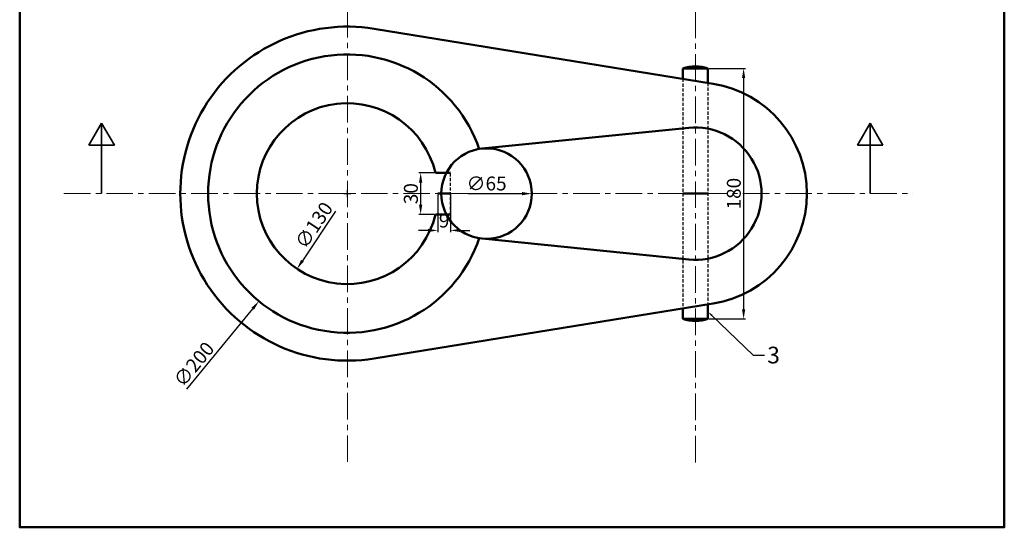
# Model space of a CAD drawing. Units: millimetres. Extents: x 1219 to 1926, y 574 to 1498.
# Tile 1 of 2: x 1219 to 1926, y 574 to 938. Entities that reach past the tile are written whole.
import ezdxf
from ezdxf import colors
from ezdxf.entities.mleader import LeaderData, LeaderLine
from ezdxf.math import Vec2, Vec3

# ---------------------------------------------------------------- set-up
doc = ezdxf.new("R2010")
doc.units = ezdxf.units.MM
doc.header["$LTSCALE"] = 0.6
doc.linetypes.add('CENTER', pattern=[50.8, 31.75, -6.35, 6.35, -6.35])
doc.linetypes.add('HIDDEN', pattern=[9.525, 6.35, -3.175])
for name, color, linetype, lineweight in [('M-CNTR', 1, 'CENTER', 18), ('M-DIMS', 2, 'Continuous', 25), ('M-HIDN', 6, 'HIDDEN', 25), ('M-OUTL', 7, 'Continuous', 50), ('M-SECT', 4, 'Continuous', 35), ('M-TEXT', 3, 'Continuous', 25), ('M-TTLB', 7, 'Continuous', 50)]:
    doc.layers.add(name, color=color, linetype=linetype, lineweight=lineweight)
doc.styles.get("Standard").update_dxf_attribs({"font": 'arial.ttf'})
doc.dimstyles.new('ISO-25', dxfattribs={"dimtxt": 10, "dimasz": 7, "dimexe": 1.25, "dimexo": 0.625, "dimtad": 1, "dimdec": 0, "dimtxsty": 'Standard', "dimcen": 2.5, "dimadec": 0, "dimazin": 0, "dimtfac": 1, "dimtdec": 0, "dimtofl": 0, "dimtmove": 0, "dimatfit": 3, "dimfxl": 1, "dimarcsym": 0})

# ---------------------------------------------------------------- blocks, each defined once
blk = doc.blocks.new('*D28')
at = {"layer": 'Defpoints', "color": 0, "ltscale": 0.6, "transparency": 16777216}
for p in [(1712.94, 903.44), (1712.94, 723.44), (1738.54, 723.44)]:
    blk.add_point(p, dxfattribs=at)
at = {"layer": 'M-DIMS', "color": 0, "lineweight": -2, "ltscale": 0.6, "transparency": 16777216}
for p, q in [((1713.57, 903.44), (1739.79, 903.44)), ((1738.54, 896.44), (1738.54, 730.44)), ((1713.57, 723.44), (1739.79, 723.44))]:
    blk.add_line(p, q, dxfattribs=at)
at = {"layer": 'M-DIMS', "color": 0, "ltscale": 0.6, "transparency": 16777216}
for points in [[(1737.37, 896.44), (1739.7, 896.44), (1738.54, 903.44)], [(1737.37, 730.44), (1739.7, 730.44), (1738.54, 723.44)]]:
    blk.add_solid(points, dxfattribs=at)
at = {"layer": 'M-DIMS', "color": 0, "ltscale": 0.6, "transparency": 16777216, "insert": (1732.8, 813.44), "char_height": 10, "attachment_point": 5, "rotation": 90}
blk.add_mtext('180', dxfattribs=at)
blk = doc.blocks.new('*D29')
at = {"layer": 'Defpoints', "color": 0, "ltscale": 0.6, "transparency": 16777216}
for p in [(1517.43, 890.7), (1390.45, 736.18)]:
    blk.add_point(p, dxfattribs=at)
at = {"layer": 'M-DIMS', "color": 0, "lineweight": -2, "ltscale": 0.6, "transparency": 16777216}
for p, q in [((1451.44, 813.44), (1456.44, 813.44)), ((1453.94, 810.94), (1453.94, 815.94)), ((1338.55, 673.02), (1386.01, 730.77))]:
    blk.add_line(p, q, dxfattribs=at)
at = {"layer": 'M-DIMS', "color": 0, "ltscale": 0.6, "transparency": 16777216}
blk.add_solid([(1385.11, 731.51), (1386.91, 730.03), (1390.45, 736.18)], dxfattribs=at)
at = {"layer": 'M-DIMS', "color": 0, "ltscale": 0.6, "transparency": 16777216, "insert": (1344.76, 690.04), "char_height": 10, "attachment_point": 5, "rotation": 50.58839}
blk.add_mtext('∅200', dxfattribs=at)
blk = doc.blocks.new('*D30')
at = {"layer": 'Defpoints', "color": 0, "ltscale": 0.6, "transparency": 16777216}
for p in [(1490.08, 867.47), (1417.8, 759.41)]:
    blk.add_point(p, dxfattribs=at)
at = {"layer": 'M-DIMS', "color": 0, "lineweight": -2, "ltscale": 0.6, "transparency": 16777216}
blk.add_line((1445.55, 800.9), (1421.7, 765.23), dxfattribs=at)
at = {"layer": 'M-DIMS', "color": 0, "ltscale": 0.6, "transparency": 16777216}
blk.add_solid([(1420.73, 765.88), (1422.67, 764.58), (1417.8, 759.41)], dxfattribs=at)
at = {"layer": 'M-DIMS', "color": 0, "ltscale": 0.6, "transparency": 16777216, "insert": (1431.05, 790.03), "char_height": 10, "attachment_point": 5, "rotation": 56.22166}
blk.add_mtext('∅130', dxfattribs=at)
blk = doc.blocks.new('*D31')
at = {"layer": 'Defpoints', "color": 0, "ltscale": 0.6, "transparency": 16777216}
for p in [(1521.44, 813.44), (1586.44, 813.44)]:
    blk.add_point(p, dxfattribs=at)
at = {"layer": 'M-DIMS', "color": 0, "lineweight": -2, "ltscale": 0.6, "transparency": 16777216}
blk.add_line((1540.68, 813.44), (1579.44, 813.44), dxfattribs=at)
at = {"layer": 'M-DIMS', "color": 0, "ltscale": 0.6, "transparency": 16777216}
blk.add_solid([(1579.44, 814.61), (1579.44, 812.27), (1586.44, 813.44)], dxfattribs=at)
at = {"layer": 'M-DIMS', "color": 0, "ltscale": 0.6, "transparency": 16777216, "insert": (1553.94, 819.45), "char_height": 10, "attachment_point": 5}
blk.add_mtext('∅65', dxfattribs=at)
blk = doc.blocks.new('*D32')
at = {"layer": 'Defpoints', "color": 0, "ltscale": 0.6, "transparency": 16777216}
for p in [(1517.19, 828.44), (1506.6, 798.44), (1517.19, 798.44)]:
    blk.add_point(p, dxfattribs=at)
at = {"layer": 'M-DIMS', "color": 0, "lineweight": -2, "ltscale": 0.6, "transparency": 16777216}
for p, q in [((1516.56, 828.44), (1505.35, 828.44)), ((1506.6, 821.44), (1506.6, 805.44)), ((1516.56, 798.44), (1505.35, 798.44))]:
    blk.add_line(p, q, dxfattribs=at)
at = {"layer": 'M-DIMS', "color": 0, "ltscale": 0.6, "transparency": 16777216}
for points in [[(1505.43, 821.44), (1507.76, 821.44), (1506.6, 828.44)], [(1505.43, 805.44), (1507.76, 805.44), (1506.6, 798.44)]]:
    blk.add_solid(points, dxfattribs=at)
at = {"layer": 'M-DIMS', "color": 0, "ltscale": 0.6, "transparency": 16777216, "insert": (1500.86, 813.44), "char_height": 10, "attachment_point": 5, "rotation": 90}
blk.add_mtext('30', dxfattribs=at)
blk = doc.blocks.new('*D33')
at = {"layer": 'Defpoints', "color": 0, "ltscale": 0.6, "transparency": 16777216}
for p in [(1518.94, 813.44), (1527.94, 813.44), (1527.94, 787.03)]:
    blk.add_point(p, dxfattribs=at)
at = {"layer": 'M-DIMS', "color": 0, "lineweight": -2, "ltscale": 0.6, "transparency": 16777216}
for p, q in [((1518.94, 812.81), (1518.94, 785.78)), ((1527.94, 812.81), (1527.94, 785.78)), ((1511.94, 787.03), (1504.94, 787.03)), ((1534.94, 787.03), (1541.94, 787.03))]:
    blk.add_line(p, q, dxfattribs=at)
at = {"layer": 'M-DIMS', "color": 0, "ltscale": 0.6, "transparency": 16777216}
for points in [[(1511.94, 788.2), (1511.94, 785.87), (1518.94, 787.03)], [(1534.94, 788.2), (1534.94, 785.87), (1527.94, 787.03)]]:
    blk.add_solid(points, dxfattribs=at)
at = {"layer": 'M-DIMS', "color": 0, "ltscale": 0.6, "transparency": 16777216, "insert": (1523.44, 792.77), "char_height": 10, "attachment_point": 5}
blk.add_mtext('9', dxfattribs=at)
blk = doc.blocks.new('SECTION-ARROW')
at = {"ltscale": 0.6}
for p, q in [((9.14, 50.7), (0, 34.87)), ((9.14, 0), (9.14, 50.7)), ((9.14, 50.7), (18.28, 34.87)), ((0, 34.87), (18.28, 34.87))]:
    blk.add_line(p, q, dxfattribs=at)

msp = doc.modelspace()

# ---------------------------------------------------------------- linework, layer by layer
at = {"layer": 'M-CNTR'}
for p, q in [((1703.94, 620.33), (1703.94, 1419.58)), ((1453.94, 620.73), (1453.94, 1146.58)), ((1250.4, 813.44), (1860.03, 813.44))]:
    msp.add_line(p, q, dxfattribs=at)
at = {"layer": 'M-HIDN', "ltscale": 0.6}
for p, q in [((1694.94, 895.94), (1694.94, 730.94)), ((1712.94, 893.02), (1712.94, 734.47)), ((1527.94, 798.44), (1527.94, 828.44))]:
    msp.add_line(p, q, dxfattribs=at)
at = {"layer": 'M-OUTL'}
for p, q in [((1473.14, 931.89), (1716.74, 892.41)), ((1473.14, 694.98), (1716.74, 734.47))]:
    msp.add_line(p, q, dxfattribs=at)
at = {"layer": 'M-OUTL', "ltscale": 0.6}
for p, q in [((1694.94, 903.44), (1694.94, 895.94)), ((1712.94, 903.44), (1694.94, 903.44)), ((1712.94, 893.02), (1712.94, 903.44)), ((1699.19, 860.7), (1550.69, 845.78)), ((1517.19, 828.44), (1527.94, 828.44)), ((1518.94, 813.44), (1527.94, 813.44)), ((1694.94, 813.44), (1712.94, 813.44)), ((1517.19, 798.44), (1527.94, 798.44)), ((1699.19, 766.18), (1550.69, 781.1)), ((1694.94, 730.94), (1694.94, 723.44)), ((1712.94, 723.44), (1712.94, 733.85)), ((1694.94, 723.44), (1712.94, 723.44))]:
    msp.add_line(p, q, dxfattribs=at)
msp.add_circle((1553.94, 813.44), 32.5, dxfattribs=at)
at = {"layer": 'M-OUTL'}
for centre, radius, start, end in [((1453.94, 813.44), 120, 80.7931, 279.2069), ((1453.94, 813.44), 100, 18.70407, 341.29593), ((1703.94, 813.44), 80, 279.2069, 80.7931), ((1453.94, 813.44), 65, 13.34236, 346.65764)]:
    msp.add_arc(centre, radius, start, end, dxfattribs=at)
at = {"layer": 'M-OUTL', "ltscale": 0.6}
for centre, radius, start, end in [((1703.94, 877.7), 27.27, 70.72588, 109.27412), ((1703.94, 813.44), 47.5, 264.26083, 95.73917), ((1703.94, 749.18), 27.27, 250.72588, 289.27412)]:
    msp.add_arc(centre, radius, start, end, dxfattribs=at)
at = {"layer": 'M-TTLB', "ltscale": 0.6}
msp.add_lwpolyline([(1218.63, 1497.51), (1925.77, 1497.51), (1925.77, 573.72), (1218.63, 573.72)], close=True, dxfattribs=at)

# ---------------------------------------------------------------- block references
at = {"layer": 'M-SECT'}
for p in [(1268.34, 813.44), (1820.28, 813.44)]:
    msp.add_blockref('SECTION-ARROW', p, dxfattribs=at)

# ---------------------------------------------------------------- dimensions: what is measured, and where the dimension line sits
at = {"layer": 'M-DIMS', "ltscale": 0.6}
for base, p1, p2, picture, middle in [((1738.54, 723.44), (1712.94, 903.44), (1712.94, 723.44), '*D28', (1732.8, 813.44)), ((1506.6, 798.44), (1517.19, 828.44), (1517.19, 798.44), '*D32', (1500.86, 813.44))]:
    dim = msp.add_linear_dim(base=base, p1=p1, p2=p2, angle=90, dimstyle='ISO-25', override={"dimclrd": 0, "dimclre": 0, "dimclrt": 0}, dxfattribs=at)
    dim.commit()
    dim.dimension.update_dxf_attribs({"geometry": picture, "text_midpoint": middle})
for p1, p2, picture, middle in [((1517.43, 890.7), (1390.45, 736.18), '*D29', (1349.41, 686.23)), ((1490.08, 867.47), (1417.8, 759.41), '*D30', (1436.05, 786.69)), ((1521.44, 813.44), (1586.44, 813.44), '*D31', (1553.94, 813.44))]:
    dim = msp.add_diameter_dim_2p(p1=p1, p2=p2, dimstyle='ISO-25', override={"dimclrd": 0, "dimclre": 0, "dimclrt": 0}, dxfattribs=at)
    dim.commit()
    dim.dimension.update_dxf_attribs({"geometry": picture, "text_midpoint": middle, "dimtype": 163})
dim = msp.add_linear_dim(base=(1527.94, 787.03), p1=(1518.94, 813.44), p2=(1527.94, 813.44), dimstyle='ISO-25', override={"dimclrd": 0, "dimclre": 0, "dimclrt": 0}, dxfattribs=at)
dim.commit()
dim.dimension.update_dxf_attribs({"geometry": '*D33', "text_midpoint": (1523.44, 792.77)})

# ---------------------------------------------------------------- leaders
at = {"layer": 'M-TEXT', "ltscale": 0.6}
ml = msp.add_multileader_mtext('Standard', dxfattribs=at)
ml.set_content('3', color=256)
ml.set_leader_properties()
ml.build(insert=Vec2(0, 0))
ctx = ml.context
ctx.base_point, ctx.char_height, ctx.plane_origin = Vec3(1753.48, 697.38), 12, Vec3(1712.94, 728.63)
notes = []
notes.append((ctx, [(0, (1, 1, 0), (1745.48, 697.38), (1, 0), 8, [(0, [(1712.94, 728.63)], 0, [])])]))
ctx.mtext.insert, ctx.mtext.flow_direction = Vec3(1755.48, 703.48), 5
for ctx, leaders in notes:
    for number, flags, end, landing, length, lines in leaders:
        leader = LeaderData()
        leader.index, (leader.has_last_leader_line, leader.has_dogleg_vector, leader.attachment_direction) = number, flags
        leader.last_leader_point, leader.dogleg_vector, leader.dogleg_length = Vec3(end), Vec3(landing), length
        for number, points, colour, breaks in lines:
            line = LeaderLine()
            line.index, line.vertices, line.color, line.breaks = number, Vec3.list(points), colors.encode_raw_color(colour), breaks
            leader.lines.append(line)
        ctx.leaders.append(leader)

doc.saveas('drawing.dxf')
